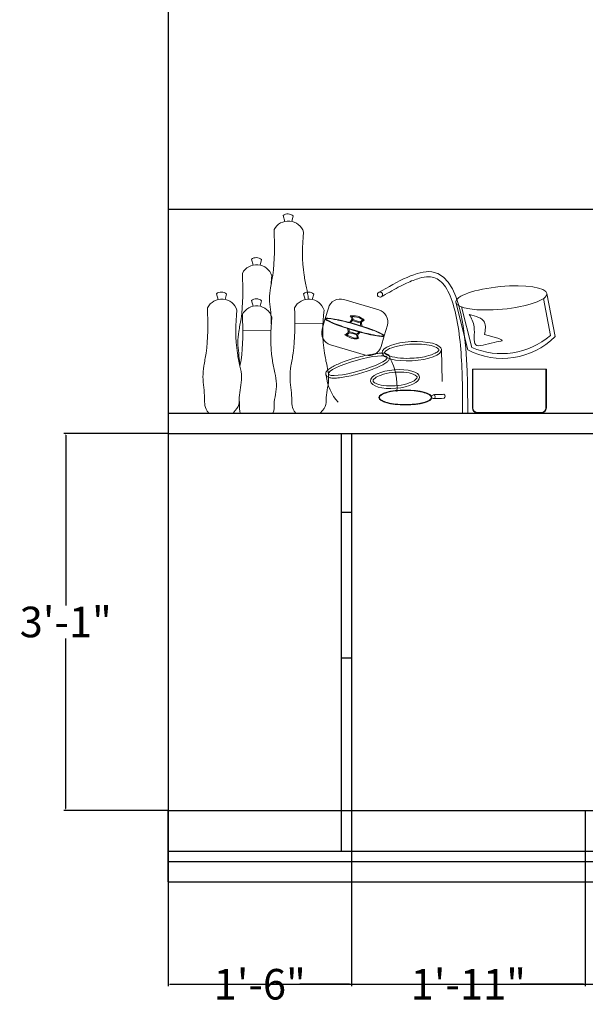
# Model space of a CAD drawing. Units: inches. Extents: x 1686244 to 1686928, y 1936095 to 1936489.
# Tile 2 of 11: x 1686248 to 1686303, y 1936338 to 1936435. Entities that reach past the tile are written whole.
import ezdxf

# ---------------------------------------------------------------- set-up
doc = ezdxf.new("R2010")
doc.units = ezdxf.units.IN
doc.header["$MEASUREMENT"] = 0
for name, color, linetype, lineweight in [('A-ANNO-DIMS', 240, 'Continuous', 18), ('A-ELEV', 7, 'Continuous', 25), ('A-FURN', 40, 'Continuous', 18)]:
    doc.layers.add(name, color=color, linetype=linetype, lineweight=lineweight)
doc.styles.get("Standard").update_dxf_attribs({"font": 'arial.ttf'})
doc.dimstyles.get("Standard").update_dxf_attribs({"dimtxt": 3, "dimasz": 0.18, "dimexe": 0.18, "dimexo": 0.0625, "dimgap": 0.09, "dimtad": 0, "dimtih": 1, "dimtoh": 1, "dimzin": 0, "dimdsep": 46, "dimlunit": 4, "dimtxsty": 'Standard', "dimcen": 0.09, "dimadec": 0, "dimazin": 0, "dimtfac": 1, "dimtofl": 0, "dimtmove": 0, "dimatfit": 3, "dimfxl": 1, "dimtolj": 1, "dimtzin": 0, "dimarcsym": 0})

# ---------------------------------------------------------------- blocks, each defined once
blk = doc.blocks.new('BO')
for p, q in [((1686271.83, 1936407.56), (1686271.656, 1936408.121)), ((1686272.51, 1936407.559), (1686272.649, 1936408.087))]:
    blk.add_line(p, q)
for centre, radius, start, end in [((1686272.133, 1936407.531), 0.759, 47.13128, 128.99703), ((1686272.168, 1936406.027), 1.569, 17.60208, 152.80615)]:
    blk.add_arc(centre, radius, start, end)
for points in [[(1686270.902, 1936396.412), (1686270.43, 1936396.902), (1686270.591, 1936398.056), (1686270.249, 1936399.621), (1686270.416, 1936401.127), (1686270.858, 1936403.218), (1686270.81, 1936405.21), (1686270.772, 1936406.745)], [(1686273.286, 1936396.412), (1686273.966, 1936397.076), (1686273.745, 1936398.056), (1686274.251, 1936399.593), (1686273.944, 1936401.127), (1686273.478, 1936403.218), (1686273.526, 1936405.21), (1686273.664, 1936406.502)]]:
    blk.add_open_spline(points, degree=3, knots=[0, 0, 0, 0, 1.54699, 3.641177, 4.739896, 6.081078, 10.57072, 10.57072, 10.57072, 10.57072])
blk = doc.blocks.new('*D87')
at = {"layer": 'A-ANNO-DIMS', "color": 0, "lineweight": -2, "transparency": 16777216}
for p, q in [((1686262.353, 1936350.349), (1686262.353, 1936340.182)), ((1686459.353, 1936350.349), (1686459.353, 1936340.182)), ((1686262.533, 1936340.362), (1686355.751, 1936340.362)), ((1686459.173, 1936340.362), (1686365.954, 1936340.362))]:
    blk.add_line(p, q, dxfattribs=at)
at = {"layer": 'A-ANNO-DIMS', "color": 0, "transparency": 16777216}
for points in [[(1686262.533, 1936340.392), (1686262.533, 1936340.332), (1686262.353, 1936340.362)], [(1686459.173, 1936340.392), (1686459.173, 1936340.332), (1686459.353, 1936340.362)]]:
    blk.add_solid(points, dxfattribs=at)
at = {"layer": 'Defpoints', "color": 0, "transparency": 16777216}
for p in [(1686262.353, 1936350.412), (1686459.353, 1936350.412), (1686459.353, 1936340.362)]:
    blk.add_point(p, dxfattribs=at)
at = {"layer": 'A-ANNO-DIMS', "color": 0, "transparency": 16777216, "insert": (1686360.853, 1936340.362), "char_height": 3, "attachment_point": 5}
blk.add_mtext('\\A1;16\'-5"', dxfattribs=at)
blk = doc.blocks.new('*D88')
at = {"layer": 'A-ANNO-DIMS', "color": 0, "lineweight": -2, "transparency": 16777216}
for p, q in [((1686262.353, 1936357.349), (1686262.353, 1936340.182)), ((1686280.343, 1936357.349), (1686280.343, 1936340.182)), ((1686262.533, 1936340.362), (1686267.412, 1936340.362)), ((1686280.163, 1936340.362), (1686275.284, 1936340.362))]:
    blk.add_line(p, q, dxfattribs=at)
at = {"layer": 'A-ANNO-DIMS', "color": 0, "transparency": 16777216}
for points in [[(1686262.533, 1936340.392), (1686262.533, 1936340.332), (1686262.353, 1936340.362)], [(1686280.163, 1936340.392), (1686280.163, 1936340.332), (1686280.343, 1936340.362)]]:
    blk.add_solid(points, dxfattribs=at)
at = {"layer": 'Defpoints', "color": 0, "transparency": 16777216}
for p in [(1686262.353, 1936357.412), (1686280.343, 1936357.412), (1686280.343, 1936340.362)]:
    blk.add_point(p, dxfattribs=at)
at = {"layer": 'A-ANNO-DIMS', "color": 0, "transparency": 16777216, "insert": (1686271.348, 1936340.362), "char_height": 3, "attachment_point": 5}
blk.add_mtext('\\A1;1\'-6"', dxfattribs=at)
blk = doc.blocks.new('*D89')
at = {"layer": 'A-ANNO-DIMS', "color": 0, "lineweight": -2, "transparency": 16777216}
for p, q in [((1686280.343, 1936357.349), (1686280.343, 1936340.182)), ((1686303.305, 1936357.351), (1686303.305, 1936340.182)), ((1686280.523, 1936340.362), (1686286.722, 1936340.362)), ((1686303.125, 1936340.362), (1686296.926, 1936340.362))]:
    blk.add_line(p, q, dxfattribs=at)
at = {"layer": 'A-ANNO-DIMS', "color": 0, "transparency": 16777216}
for points in [[(1686280.523, 1936340.392), (1686280.523, 1936340.332), (1686280.343, 1936340.362)], [(1686303.125, 1936340.392), (1686303.125, 1936340.332), (1686303.305, 1936340.362)]]:
    blk.add_solid(points, dxfattribs=at)
at = {"layer": 'Defpoints', "color": 0, "transparency": 16777216}
for p in [(1686280.343, 1936357.412), (1686303.305, 1936357.414), (1686303.305, 1936340.362)]:
    blk.add_point(p, dxfattribs=at)
at = {"layer": 'A-ANNO-DIMS', "color": 0, "transparency": 16777216, "insert": (1686291.824, 1936340.362), "char_height": 3, "attachment_point": 5}
blk.add_mtext('\\A1;1\'-11"', dxfattribs=at)
blk = doc.blocks.new('*D96')
at = {"layer": 'A-ANNO-DIMS', "color": 0, "lineweight": -2, "transparency": 16777216}
for p, q in [((1686262.29, 1936394.412), (1686252.123, 1936394.412)), ((1686252.303, 1936394.232), (1686252.303, 1936377.535)), ((1686252.303, 1936357.592), (1686252.303, 1936374.289)), ((1686262.29, 1936357.412), (1686252.123, 1936357.412))]:
    blk.add_line(p, q, dxfattribs=at)
at = {"layer": 'A-ANNO-DIMS', "color": 0, "transparency": 16777216}
for points in [[(1686252.273, 1936394.232), (1686252.333, 1936394.232), (1686252.303, 1936394.412)], [(1686252.273, 1936357.592), (1686252.333, 1936357.592), (1686252.303, 1936357.412)]]:
    blk.add_solid(points, dxfattribs=at)
at = {"layer": 'Defpoints', "color": 0, "transparency": 16777216}
for p in [(1686262.353, 1936394.412), (1686252.303, 1936357.412), (1686262.353, 1936357.412)]:
    blk.add_point(p, dxfattribs=at)
at = {"layer": 'A-ANNO-DIMS', "color": 0, "transparency": 16777216, "insert": (1686252.303, 1936375.912), "char_height": 3, "attachment_point": 5}
blk.add_mtext('\\A1;3\'-1"', dxfattribs=at)

msp = doc.modelspace()

# ---------------------------------------------------------------- linework, layer by layer
at = {"layer": 'A-ELEV'}
for p, q in [((1686262.353, 1936416.412), (1686341.693, 1936416.412)), ((1686262.353, 1936396.412), (1686341.687, 1936396.414)), ((1686262.353, 1936394.412), (1686341.693, 1936394.414)), ((1686279.343, 1936394.412), (1686279.343, 1936353.412)), ((1686280.343, 1936394.412), (1686280.343, 1936357.412)), ((1686279.343, 1936386.698), (1686280.343, 1936386.698)), ((1686279.343, 1936372.383), (1686280.343, 1936372.383)), ((1686262.353, 1936350.412), (1686262.353, 1936357.412)), ((1686262.353, 1936353.412), (1686459.353, 1936353.412)), ((1686262.353, 1936352.412), (1686459.353, 1936352.412)), ((1686262.353, 1936350.412), (1686459.353, 1936350.412))]:
    msp.add_line(p, q, dxfattribs=at)
msp.add_lwpolyline([(1686459.353, 1936357.412), (1686459.353, 1936467.412), (1686262.353, 1936467.412), (1686262.353, 1936357.412)], close=True, dxfattribs=at)
at = {"layer": 'A-FURN'}
for p, q in [((1686273.815, 1936415.226), (1686273.641, 1936415.787)), ((1686274.495, 1936415.225), (1686274.634, 1936415.753)), ((1686270.703, 1936410.938), (1686270.529, 1936411.499)), ((1686271.383, 1936410.938), (1686271.522, 1936411.466)), ((1686275.82, 1936407.56), (1686275.646, 1936408.121)), ((1686299.535, 1936408.137), (1686300.337, 1936403.923)), ((1686270.703, 1936406.896), (1686270.529, 1936407.457)), ((1686271.383, 1936406.895), (1686271.522, 1936407.424)), ((1686276.5, 1936407.559), (1686276.64, 1936408.087)), ((1686299.188, 1936407.647), (1686299.88, 1936404.009)), ((1686274.79, 1936405.235), (1686277.516, 1936405.21)), ((1686269.675, 1936404.47), (1686272.399, 1936404.547)), ((1686289.18, 1936402.69), (1686289.251, 1936399.511)), ((1686292.226, 1936400.731), (1686299.484, 1936400.731)), ((1686292.226, 1936400.731), (1686292.226, 1936396.915)), ((1686292.276, 1936400.731), (1686292.276, 1936396.915)), ((1686299.434, 1936400.731), (1686299.434, 1936396.915)), ((1686299.484, 1936400.731), (1686299.484, 1936396.915)), ((1686292.726, 1936396.465), (1686298.984, 1936396.465)), ((1686292.726, 1936396.415), (1686298.984, 1936396.415))]:
    msp.add_line(p, q, dxfattribs=at)
for points in [[(1686277.776, 1936405.677), (1686278.082, 1936406.721, -0.414214), (1686279.603, 1936407.553), (1686283.041, 1936406.547, -0.414214), (1686283.873, 1936405.025), (1686283.567, 1936403.981)], [(1686277.776, 1936405.677), (1686277.47, 1936404.632, 0.414214), (1686278.303, 1936403.111), (1686281.74, 1936402.104, 0.414214), (1686283.262, 1936402.937), (1686283.567, 1936403.981)]]:
    msp.add_lwpolyline(points, format="xyb", dxfattribs=at)
for points in [[(1686290.586, 1936407.29), (1686291.772, 1936402.616)], [(1686291.151, 1936406.822), (1686292.158, 1936402.855)]]:
    msp.add_lwpolyline(points, dxfattribs=at)
msp.add_circle((1686283.152, 1936408.039), 0.25, dxfattribs=at)
for centre, radius, start, end in [((1686274.118, 1936415.197), 0.759, 47.13128, 128.99703), ((1686274.153, 1936413.694), 1.569, 17.60208, 152.80615), ((1686271.006, 1936410.91), 0.759, 47.13128, 128.99703), ((1686271.041, 1936409.406), 1.569, 17.60208, 152.80615), ((1686276.124, 1936407.531), 0.759, 47.13128, 128.99703), ((1686271.006, 1936406.868), 0.759, 47.13128, 128.99703), ((1686276.159, 1936406.027), 1.569, 17.60208, 152.80615), ((1686271.041, 1936405.364), 1.569, 17.60208, 152.80615), ((1686281.77, 1936408.493), 3.273, 246.06969, 260.59906), ((1686281.77, 1936408.493), 3.177, 246.09715, 260.54093), ((1686279.621, 1936401.151), 3.177, 66.8207, 81.26447), ((1686279.621, 1936401.151), 3.273, 66.76257, 81.29193), ((1686295.173, 1936409.043), 7.272, 242.10987, 315.24217), ((1686295.097, 1936409.603), 7.36, 246.46572, 310.535), ((1686279.391, 1936399.123), 5.435, 353.73815, 29.7733), ((1686282.462, 1936400.584), 4.621, 185.86891, 222.35988), ((1686292.726, 1936396.915), 0.5, 180, 270), ((1686292.726, 1936396.915), 0.45, 180, 270), ((1686298.984, 1936396.915), 0.5, 270, 0), ((1686298.984, 1936396.915), 0.45, 270, 0)]:
    msp.add_arc(centre, radius, start, end, dxfattribs=at)
for centre, major_axis, ratio in [((1686295.061, 1936407.713), (-4.475, -0.423), 0.247704), ((1686280.672, 1936404.829), (-2.896, 0.848), 0.103756), ((1686286.271, 1936402.484), (-2.916, -0.153), 0.322421), ((1686280.969, 1936401.063), (-2.882, -0.818), 0.180882), ((1686284.628, 1936399.751), (-2.412, -0.199), 0.37765), ((1686285.641, 1936397.94), (-2.592, 0), 0.283655)]:
    msp.add_ellipse(centre, major_axis=major_axis, ratio=ratio, dxfattribs=at)
msp.add_ellipse((1686288.398, 1936398.007), major_axis=(0, 0.181), ratio=0.973714, start_param=-3.141592653589793, end_param=3.141592653589793, dxfattribs=at)
for points, knots in [([(1686272.477, 1936405.173), (1686272.475, 1936405.301), (1686272.494, 1936406.101), (1686272.234, 1936407.287), (1686272.401, 1936408.793), (1686272.844, 1936410.884), (1686272.796, 1936412.877), (1686272.757, 1936414.411)], [1.147862, 1.147862, 1.147862, 1.147862, 1.54699, 3.641177, 4.739896, 6.081078, 10.57072, 10.57072, 10.57072, 10.57072]), ([(1686276.103, 1936407.596), (1686276.103, 1936407.598), (1686276.095, 1936407.966), (1686275.929, 1936408.793), (1686275.463, 1936410.884), (1686275.511, 1936412.877), (1686275.649, 1936414.168)], [3.635922, 3.635922, 3.635922, 3.635922, 3.641177, 4.739896, 6.081078, 10.57072, 10.57072, 10.57072, 10.57072]), ([(1686269.364, 1936401.219), (1686269.364, 1936401.236), (1686269.357, 1936401.928), (1686269.122, 1936402.999), (1686269.289, 1936404.506), (1686269.732, 1936406.596), (1686269.684, 1936408.589), (1686269.646, 1936410.123)], [1.494459, 1.494459, 1.494459, 1.494459, 1.54699, 3.641177, 4.739896, 6.081078, 10.57072, 10.57072, 10.57072, 10.57072]), ([(1686282.989, 1936408.235), (1686284.915, 1936409.337), (1686291.743, 1936413.244), (1686291.76, 1936401.207), (1686291.76, 1936396.412)], [0, 0, 0, 0, 5.61681, 19.92146, 19.92146, 19.92146, 19.92146]), ([(1686283.238, 1936407.801), (1686283.527, 1936407.967), (1686283.816, 1936408.132), (1686284.673, 1936408.613), (1686285.231, 1936408.913), (1686286.206, 1936409.366), (1686286.631, 1936409.534), (1686287.349, 1936409.736), (1686287.65, 1936409.786), (1686288.173, 1936409.792), (1686288.39, 1936409.749), (1686288.801, 1936409.577), (1686288.993, 1936409.447), (1686289.362, 1936409.089), (1686289.537, 1936408.861), (1686290.019, 1936408.048), (1686290.285, 1936407.336), (1686290.704, 1936405.693), (1686290.858, 1936404.765), (1686291.191, 1936401.855), (1686291.244, 1936399.745), (1686291.259, 1936397.472), (1686291.26, 1936397.036), (1686291.26, 1936396.553), (1686291.26, 1936396.482), (1686291.26, 1936396.412)], [0, 0, 0, 0, 0.845661, 0.845661, 2.536984, 2.536984, 3.971688, 3.971688, 5.199268, 5.199268, 6.426848, 6.426848, 7.654428, 7.654428, 8.882008, 8.882008, 11.295285, 11.295285, 13.708562, 13.708562, 18.511781, 18.511781, 19.712349, 19.712349, 19.92162, 19.92162, 19.92162, 19.92162]), ([(1686274.893, 1936396.412), (1686274.421, 1936396.902), (1686274.582, 1936398.056), (1686274.24, 1936399.621), (1686274.406, 1936401.127), (1686274.849, 1936403.218), (1686274.801, 1936405.21), (1686274.763, 1936406.745)], [0, 0, 0, 0, 1.54699, 3.641177, 4.739896, 6.081078, 10.57072, 10.57072, 10.57072, 10.57072]), ([(1686277.276, 1936396.412), (1686277.956, 1936397.076), (1686277.736, 1936398.056), (1686278.242, 1936399.593), (1686277.934, 1936401.127), (1686277.468, 1936403.218), (1686277.516, 1936405.21), (1686277.655, 1936406.502)], [0, 0, 0, 0, 1.54699, 3.641177, 4.739896, 6.081078, 10.57072, 10.57072, 10.57072, 10.57072]), ([(1686269.406, 1936401.021), (1686269.442, 1936401.219), (1686269.726, 1936402.792), (1686269.684, 1936404.547), (1686269.646, 1936406.081)], [5.437611, 5.437611, 5.437611, 5.437611, 6.081078, 10.57072, 10.57072, 10.57072, 10.57072]), ([(1686272.647, 1936396.412), (1686272.784, 1936396.733), (1686272.681, 1936397.582), (1686273.124, 1936398.929), (1686272.817, 1936400.463), (1686272.351, 1936402.554), (1686272.399, 1936404.547), (1686272.537, 1936405.838)], [0.586481, 0.586481, 0.586481, 0.586481, 1.54699, 3.641177, 4.739896, 6.081078, 10.57072, 10.57072, 10.57072, 10.57072]), ([(1686277.805, 1936405.668), (1686277.804, 1936405.667), (1686277.804, 1936405.661), (1686277.823, 1936405.634), (1686277.842, 1936405.616), (1686277.931, 1936405.547), (1686278.037, 1936405.486), (1686278.489, 1936405.267), (1686278.974, 1936405.079), (1686280.107, 1936404.696), (1686280.753, 1936404.503), (1686281.833, 1936404.22), (1686282.284, 1936404.116), (1686283.008, 1936403.982), (1686283.283, 1936403.952), (1686283.481, 1936403.964), (1686283.517, 1936403.974), (1686283.54, 1936403.988), (1686283.539, 1936403.988), (1686283.539, 1936403.993), (1686283.536, 1936404.003), (1686283.512, 1936404.032), (1686283.492, 1936404.05), (1686283.393, 1936404.123), (1686283.27, 1936404.192), (1686282.804, 1936404.409), (1686282.361, 1936404.58), (1686281.335, 1936404.929), (1686280.753, 1936405.106), (1686279.634, 1936405.409), (1686279.1, 1936405.534), (1686278.268, 1936405.687), (1686277.969, 1936405.713), (1686277.826, 1936405.684), (1686277.811, 1936405.675), (1686277.805, 1936405.669), (1686277.805, 1936405.669), (1686277.805, 1936405.668)], [0, 0, 0, 0, 0.129873, 0.129873, 0.259747, 0.259747, 0.557497, 0.557497, 1.196564, 1.196564, 1.835631, 1.835631, 2.348435, 2.348435, 2.861238, 2.861238, 3.048242, 3.048242, 3.170903, 3.170903, 3.293565, 3.293565, 3.416226, 3.416226, 3.737883, 3.737883, 4.321058, 4.321058, 4.904233, 4.904233, 5.496223, 5.496223, 6.088213, 6.088213, 6.228874, 6.228874, 6.283185, 6.283185, 6.283185, 6.283185]), ([(1686280.148, 1936405.301), (1686280.3, 1936405.458), (1686280.392, 1936405.581), (1686280.403, 1936405.687), (1686280.394, 1936405.713), (1686280.344, 1936405.785), (1686280.322, 1936405.812), (1686280.235, 1936405.941)], [0, 0, 0, 0, 0.1303544, 0.1303544, 0.1938501, 0.1938501, 0.2257011, 0.2257011, 0.2257011, 0.2257011]), ([(1686280.235, 1936405.941), (1686280.631, 1936406.006), (1686280.892, 1936405.935), (1686281.278, 1936405.798), (1686281.418, 1936405.715), (1686281.589, 1936405.526)], [0, 0, 0, 0, 0.2296311, 0.2296311, 0.3676138, 0.3676138, 0.3676138, 0.3676138]), ([(1686280.262, 1936405.269), (1686280.396, 1936405.422), (1686280.586, 1936405.641), (1686280.422, 1936405.841), (1686280.373, 1936405.901)], [0, 0, 0, 0, 0.5043831, 0.7188071, 0.7188071, 0.7188071, 0.7188071]), ([(1686280.373, 1936405.901), (1686280.719, 1936405.859), (1686281.12, 1936405.81), (1686281.439, 1936405.583), (1686281.483, 1936405.552)], [0, 0, 0, 0, 1.010877, 1.170767, 1.170767, 1.170767, 1.170767]), ([(1686281.281, 1936404.979), (1686281.236, 1936405.163), (1686281.184, 1936405.424), (1686281.41, 1936405.522), (1686281.481, 1936405.553)], [0.0103618, 0.0103618, 0.0103618, 0.0103618, 0.1583733, 0.2257011, 0.2257011, 0.2257011, 0.2257011]), ([(1686281.389, 1936404.948), (1686281.343, 1936405.131), (1686281.322, 1936405.251), (1686281.346, 1936405.362), (1686281.358, 1936405.381), (1686281.434, 1936405.428), (1686281.475, 1936405.446), (1686281.589, 1936405.526)], [0.0103618, 0.0103618, 0.0103618, 0.0103618, 0.1154664, 0.1154664, 0.1835905, 0.1835905, 0.2257011, 0.2257011, 0.2257011, 0.2257011]), ([(1686291.908, 1936406.091), (1686292.119, 1936405.723), (1686292.615, 1936404.857), (1686292.079, 1936402.496), (1686293.91, 1936403.352), (1686295.78, 1936403.505), (1686294.389, 1936403.859), (1686293.411, 1936404.107)], [0, 0, 0, 0, 1.30809, 3.075407, 4.908589, 5.676466, 7.489736, 7.489736, 7.489736, 7.489736]), ([(1686293.411, 1936404.107), (1686293.487, 1936404.559), (1686293.667, 1936405.636), (1686292.556, 1936405.922), (1686291.91, 1936406.088)], [0, 0, 0, 0, 1.215664, 2.901036, 2.901036, 2.901036, 2.901036]), ([(1686279.976, 1936404.714), (1686280.02, 1936404.499), (1686280.031, 1936404.346), (1686279.983, 1936404.251), (1686279.961, 1936404.234), (1686279.88, 1936404.2), (1686279.847, 1936404.189), (1686279.704, 1936404.128)], [0, 0, 0, 0, 0.1303544, 0.1303544, 0.1938501, 0.1938501, 0.2257011, 0.2257011, 0.2257011, 0.2257011]), ([(1686280.09, 1936404.679), (1686280.119, 1936404.478), (1686280.162, 1936404.191), (1686279.915, 1936404.111), (1686279.842, 1936404.087)], [0, 0, 0, 0, 0.5043831, 0.7188071, 0.7188071, 0.7188071, 0.7188071]), ([(1686281.104, 1936404.373), (1686280.967, 1936404.243), (1686280.782, 1936404.051), (1686280.92, 1936403.846), (1686280.963, 1936403.782)], [0.0103618, 0.0103618, 0.0103618, 0.0103618, 0.1583733, 0.2257011, 0.2257011, 0.2257011, 0.2257011]), ([(1686281.211, 1936404.342), (1686281.074, 1936404.213), (1686280.992, 1936404.122), (1686280.952, 1936404.016), (1686280.952, 1936403.994), (1686280.991, 1936403.913), (1686281.015, 1936403.876), (1686281.068, 1936403.747)], [0.0103618, 0.0103618, 0.0103618, 0.0103618, 0.1154664, 0.1154664, 0.1835905, 0.1835905, 0.2257011, 0.2257011, 0.2257011, 0.2257011]), ([(1686279.704, 1936404.128), (1686280.003, 1936403.859), (1686280.261, 1936403.779), (1686280.659, 1936403.686), (1686280.822, 1936403.68), (1686281.068, 1936403.747)], [0, 0, 0, 0, 0.2296311, 0.2296311, 0.3676138, 0.3676138, 0.3676138, 0.3676138]), ([(1686279.842, 1936404.087), (1686280.156, 1936403.936), (1686280.52, 1936403.761), (1686280.911, 1936403.78), (1686280.964, 1936403.782)], [0, 0, 0, 0, 1.010877, 1.170767, 1.170767, 1.170767, 1.170767]), ([(1686283.605, 1936402.344), (1686283.605, 1936402.333), (1686283.608, 1936402.32), (1686283.643, 1936402.268), (1686283.678, 1936402.231), (1686283.789, 1936402.152), (1686283.864, 1936402.11), (1686284.176, 1936401.977), (1686284.492, 1936401.895), (1686285.233, 1936401.794), (1686285.657, 1936401.773), (1686286.652, 1936401.8), (1686287.227, 1936401.873), (1686288.059, 1936402.072), (1686288.36, 1936402.18), (1686288.71, 1936402.364), (1686288.81, 1936402.438), (1686288.909, 1936402.543), (1686288.928, 1936402.579), (1686288.941, 1936402.619), (1686288.94, 1936402.625), (1686288.929, 1936402.657), (1686288.914, 1936402.686), (1686288.834, 1936402.762), (1686288.772, 1936402.806), (1686288.521, 1936402.935), (1686288.274, 1936403.017), (1686287.673, 1936403.134), (1686287.321, 1936403.171), (1686286.37, 1936403.201), (1686285.745, 1936403.155), (1686284.764, 1936402.977), (1686284.379, 1936402.864), (1686283.931, 1936402.663), (1686283.801, 1936402.582), (1686283.66, 1936402.459), (1686283.628, 1936402.413), (1686283.605, 1936402.363), (1686283.604, 1936402.353), (1686283.605, 1936402.344)], [0, 0, 0, 0, 0.193033, 0.193033, 0.386066, 0.386066, 0.579098, 0.579098, 1.036223, 1.036223, 1.493347, 1.493347, 2.091015, 2.091015, 2.531383, 2.531383, 2.814347, 2.814347, 3.022047, 3.022047, 3.229746, 3.229746, 3.437445, 3.437445, 3.645144, 3.645144, 4.05192, 4.05192, 4.458696, 4.458696, 5.088556, 5.088556, 5.589787, 5.589787, 5.892877, 5.892877, 6.117294, 6.117294, 6.283185, 6.283185, 6.283185, 6.283185]), ([(1686277.847, 1936400.177), (1686277.865, 1936400.111), (1686277.904, 1936400.054), (1686277.989, 1936399.973), (1686278.034, 1936399.946), (1686278.126, 1936399.905), (1686278.172, 1936399.891), (1686278.341, 1936399.852), (1686278.476, 1936399.842), (1686278.792, 1936399.844), (1686278.973, 1936399.856), (1686279.62, 1936399.93), (1686280.166, 1936400.036), (1686281.293, 1936400.322), (1686281.872, 1936400.502), (1686282.785, 1936400.843), (1686283.144, 1936401.001), (1686283.578, 1936401.237), (1686283.709, 1936401.319), (1686283.894, 1936401.462), (1686283.959, 1936401.523), (1686284.047, 1936401.643), (1686284.078, 1936401.698), (1686284.108, 1936401.822), (1686284.109, 1936401.89), (1686284.072, 1936402.017), (1686284.034, 1936402.072), (1686283.952, 1936402.152), (1686283.907, 1936402.179), (1686283.818, 1936402.22), (1686283.772, 1936402.234), (1686283.607, 1936402.273), (1686283.474, 1936402.284), (1686283.164, 1936402.283), (1686282.988, 1936402.272), (1686282.353, 1936402.202), (1686281.817, 1936402.1), (1686280.705, 1936401.822), (1686280.131, 1936401.646), (1686279.202, 1936401.304), (1686278.828, 1936401.142), (1686278.379, 1936400.901), (1686278.244, 1936400.818), (1686278.054, 1936400.672), (1686277.986, 1936400.611), (1686277.895, 1936400.49), (1686277.864, 1936400.436), (1686277.831, 1936400.311), (1686277.828, 1936400.242), (1686277.847, 1936400.177)], [0, 0, 0, 0, 0.105893, 0.105893, 0.211786, 0.211786, 0.317679, 0.317679, 0.576196, 0.576196, 0.834713, 0.834713, 1.414893, 1.414893, 1.995073, 1.995073, 2.461973, 2.461973, 2.72225, 2.72225, 2.914346, 2.914346, 3.039937, 3.039937, 3.143354, 3.143354, 3.246771, 3.246771, 3.350188, 3.350188, 3.453605, 3.453605, 3.709337, 3.709337, 3.965069, 3.965069, 4.5386, 4.5386, 5.112131, 5.112131, 5.590821, 5.590821, 5.854021, 5.854021, 6.049742, 6.049742, 6.177036, 6.177036, 6.283185, 6.283185, 6.283185, 6.283185]), ([(1686282.465, 1936399.573), (1686282.466, 1936399.554), (1686282.472, 1936399.534), (1686282.515, 1936399.473), (1686282.555, 1936399.433), (1686282.675, 1936399.351), (1686282.755, 1936399.309), (1686283.082, 1936399.181), (1686283.409, 1936399.112), (1686284.146, 1936399.056), (1686284.556, 1936399.067), (1686285.344, 1936399.167), (1686285.722, 1936399.256), (1686286.273, 1936399.458), (1686286.473, 1936399.565), (1686286.687, 1936399.732), (1686286.741, 1936399.796), (1686286.788, 1936399.88), (1686286.792, 1936399.905), (1686286.791, 1936399.943), (1686286.787, 1936399.962), (1686286.747, 1936400.022), (1686286.709, 1936400.063), (1686286.59, 1936400.146), (1686286.508, 1936400.19), (1686286.182, 1936400.319), (1686285.86, 1936400.388), (1686285.131, 1936400.446), (1686284.724, 1936400.436), (1686283.941, 1936400.34), (1686283.564, 1936400.254), (1686283.002, 1936400.053), (1686282.796, 1936399.945), (1686282.574, 1936399.775), (1686282.518, 1936399.71), (1686282.466, 1936399.619), (1686282.463, 1936399.594), (1686282.465, 1936399.573)], [0, 0, 0, 0, 0.218372, 0.218372, 0.436745, 0.436745, 0.655117, 0.655117, 1.170938, 1.170938, 1.686759, 1.686759, 2.20258, 2.20258, 2.618678, 2.618678, 2.894855, 2.894855, 3.119413, 3.119413, 3.343972, 3.343972, 3.56853, 3.56853, 3.793089, 3.793089, 4.304895, 4.304895, 4.816702, 4.816702, 5.328508, 5.328508, 5.75235, 5.75235, 6.030072, 6.030072, 6.283185, 6.283185, 6.283185, 6.283185]), ([(1686283.089, 1936397.94), (1686283.089, 1936397.876), (1686283.126, 1936397.808), (1686283.293, 1936397.667), (1686283.421, 1936397.597), (1686283.96, 1936397.395), (1686284.527, 1936397.294), (1686285.757, 1936397.225), (1686286.416, 1936397.257), (1686287.393, 1936397.421), (1686287.75, 1936397.533), (1686288.095, 1936397.74), (1686288.169, 1936397.824), (1686288.205, 1936397.974), (1686288.176, 1936398.05), (1686287.995, 1936398.213), (1686287.843, 1936398.294), (1686287.251, 1936398.502), (1686286.671, 1936398.598), (1686285.427, 1936398.654), (1686284.77, 1936398.615), (1686283.829, 1936398.443), (1686283.496, 1936398.332), (1686283.178, 1936398.132), (1686283.111, 1936398.052), (1686283.09, 1936397.967), (1686283.089, 1936397.954), (1686283.089, 1936397.94)], [0, 0, 0, 0, 0.323549, 0.323549, 0.647097, 0.647097, 1.376352, 1.376352, 2.105606, 2.105606, 2.698637, 2.698637, 3.072846, 3.072846, 3.447055, 3.447055, 3.821265, 3.821265, 4.553416, 4.553416, 5.285566, 5.285566, 5.858503, 5.858503, 6.21544, 6.21544, 6.283185, 6.283185, 6.283185, 6.283185]), ([(1686269.41, 1936396.412), (1686269.35, 1936396.682), (1686269.381, 1936397.134), (1686269.348, 1936397.594), (1686269.33, 1936397.779)], [0.697318, 0.697318, 0.697318, 0.697318, 1.54699, 2.113046, 2.113046, 2.113046, 2.113046]), ([(1686288.385, 1936398.187), (1686288.544, 1936398.243), (1686288.799, 1936398.245), (1686289.141, 1936398.236), (1686289.318, 1936398.254), (1686289.403, 1936398.265)], [0, 0, 0, 0, 0.916458, 1.428142, 1.911036, 1.911036, 1.911036, 1.911036]), ([(1686289.403, 1936398.265), (1686289.49, 1936398.202), (1686289.573, 1936398.076), (1686289.52, 1936397.932), (1686289.463, 1936397.861)], [0.0418453, 0.0418453, 0.0418453, 0.0418453, 0.5382692, 0.9735226, 0.9735226, 0.9735226, 0.9735226])]:
    msp.add_open_spline(points, degree=3, knots=knots, dxfattribs=at)
for points in [[(1686272.467, 1936409.068), (1686272.485, 1936409.347), (1686272.509, 1936409.619), (1686272.537, 1936409.88)], [(1686288.385, 1936397.826), (1686288.744, 1936397.843), (1686289.103, 1936397.861), (1686289.463, 1936397.861)]]:
    msp.add_open_spline(points, degree=3, dxfattribs=at)

# ---------------------------------------------------------------- block references
msp.add_blockref('BO', (-4.556, 0), dxfattribs=at)

# ---------------------------------------------------------------- dimensions: what is measured, and where the dimension line sits
at = {"layer": 'A-ANNO-DIMS'}
dim = msp.add_linear_dim(base=(1686252.303, 1936357.412), p1=(1686262.353, 1936394.412), p2=(1686262.353, 1936357.412), angle=90, dimstyle='Standard', override={"dimdec": 1, "dimlfac": 1, "dimrnd": 0, "dimzin": 1, "dimdsep": 46, "dimlunit": 4, "dimfrac": 2}, dxfattribs=at)
dim.commit()
dim.dimension.update_dxf_attribs({"geometry": '*D96', "text_midpoint": (1686252.303, 1936375.912)})
for base, p1, p2, picture, middle in [((1686280.343, 1936340.362), (1686262.353, 1936357.412), (1686280.343, 1936357.412), '*D88', (1686271.348, 1936340.362)), ((1686303.305, 1936340.362), (1686280.343, 1936357.412), (1686303.305, 1936357.414), '*D89', (1686291.824, 1936340.362)), ((1686459.353, 1936340.362), (1686262.353, 1936350.412), (1686459.353, 1936350.412), '*D87', (1686360.853, 1936340.362))]:
    dim = msp.add_linear_dim(base=base, p1=p1, p2=p2, dimstyle='Standard', override={"dimdec": 1, "dimlfac": 1, "dimrnd": 0, "dimzin": 1, "dimdsep": 46, "dimlunit": 4, "dimfrac": 2}, dxfattribs=at)
    dim.commit()
    dim.dimension.update_dxf_attribs({"geometry": picture, "text_midpoint": middle})

doc.saveas('drawing.dxf')
